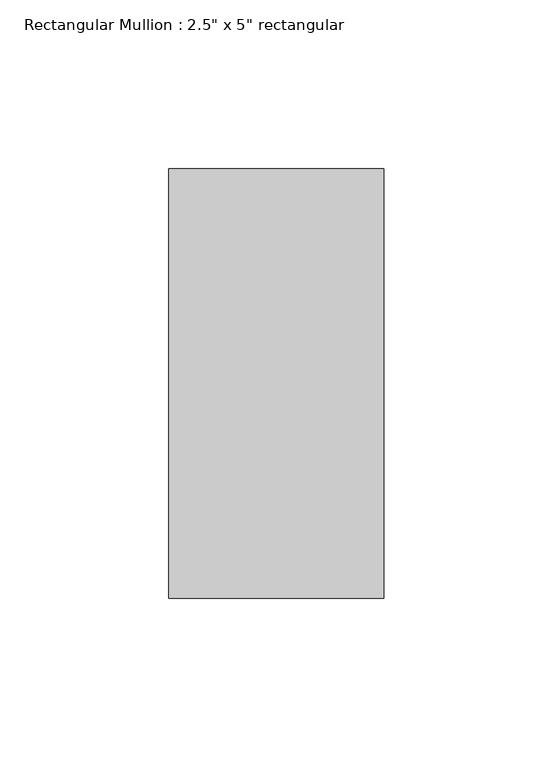
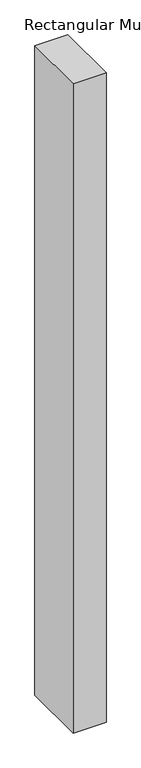
"""IFC4 building model written with IfcOpenShell, lengths in millimetres: member geometry."""

from ifc_helpers import new_model, si_unit, frame, origin, place, context, project, spatial, polyline, outline, extrude, source, transform, mapped, element, save


def member_ef344e51(model_context):
    return source(origin(), model_context, "Body", "SweptSolid", [
        extrude(outline(polyline([(0.0, 63.5), (0.0, -63.5), (-63.5, -63.5), (-63.5, 63.5), (0.0, 63.5)])), frame((0.0, 0.0, -1319.931705), z_axis=(0.0, 0.0, 1.0), x_axis=(1.0, 0.0, 0.0)), (0.0, 0.0, 1.0), 1319.931705),
    ])


if __name__ == "__main__":
    model = new_model("IFC4")
    model_context = context("Model", 3, world=origin())
    ifc_project = project(units=[si_unit("LENGTHUNIT", "METRE", prefix="MILLI")], contexts=[model_context])
    site = spatial("IfcSite", under=ifc_project)
    building = spatial("IfcBuilding", under=site)
    placement = place(None, origin())
    member_shape = member_ef344e51(model_context)
    element("IfcMember", 1, ObjectType="Rectangular Mullion : 2.5\" x 5\" rectangular", at=placement, inside=building, context=model_context, shape_type="MappedRepresentation", body=[
        mapped(member_shape, transform((0.0, 0.0, 0.0), x_axis=(1.0, 0.0, 0.0), y_axis=(0.0, 1.0, 0.0), z_axis=(0.0, 0.0, 1.0))),
    ])
    save(model, "model.ifc")

# Revit data of these elements
# Type "Rectangular Mullion : 2.5\" x 5\" rectangular"
#   built-in parameter 1007304 = 0.416667 (stored number, unit not read)
#   built-in parameter 1007301 = 0.104167 (stored number, unit not read)
#   built-in parameter 1007300 = 0.104167 (stored number, unit not read)
# Element 1 (IfcMember, "Rectangular Mullion : 2.5\" x 5\" rectangular")
#   Materials on its faces: "Iron, Ductile"
# Materials
#   "Iron, Ductile": class "Metal", colour RGB 0 0 0, transparency 0, Description = "Ductile cast iron", Cost = 0
